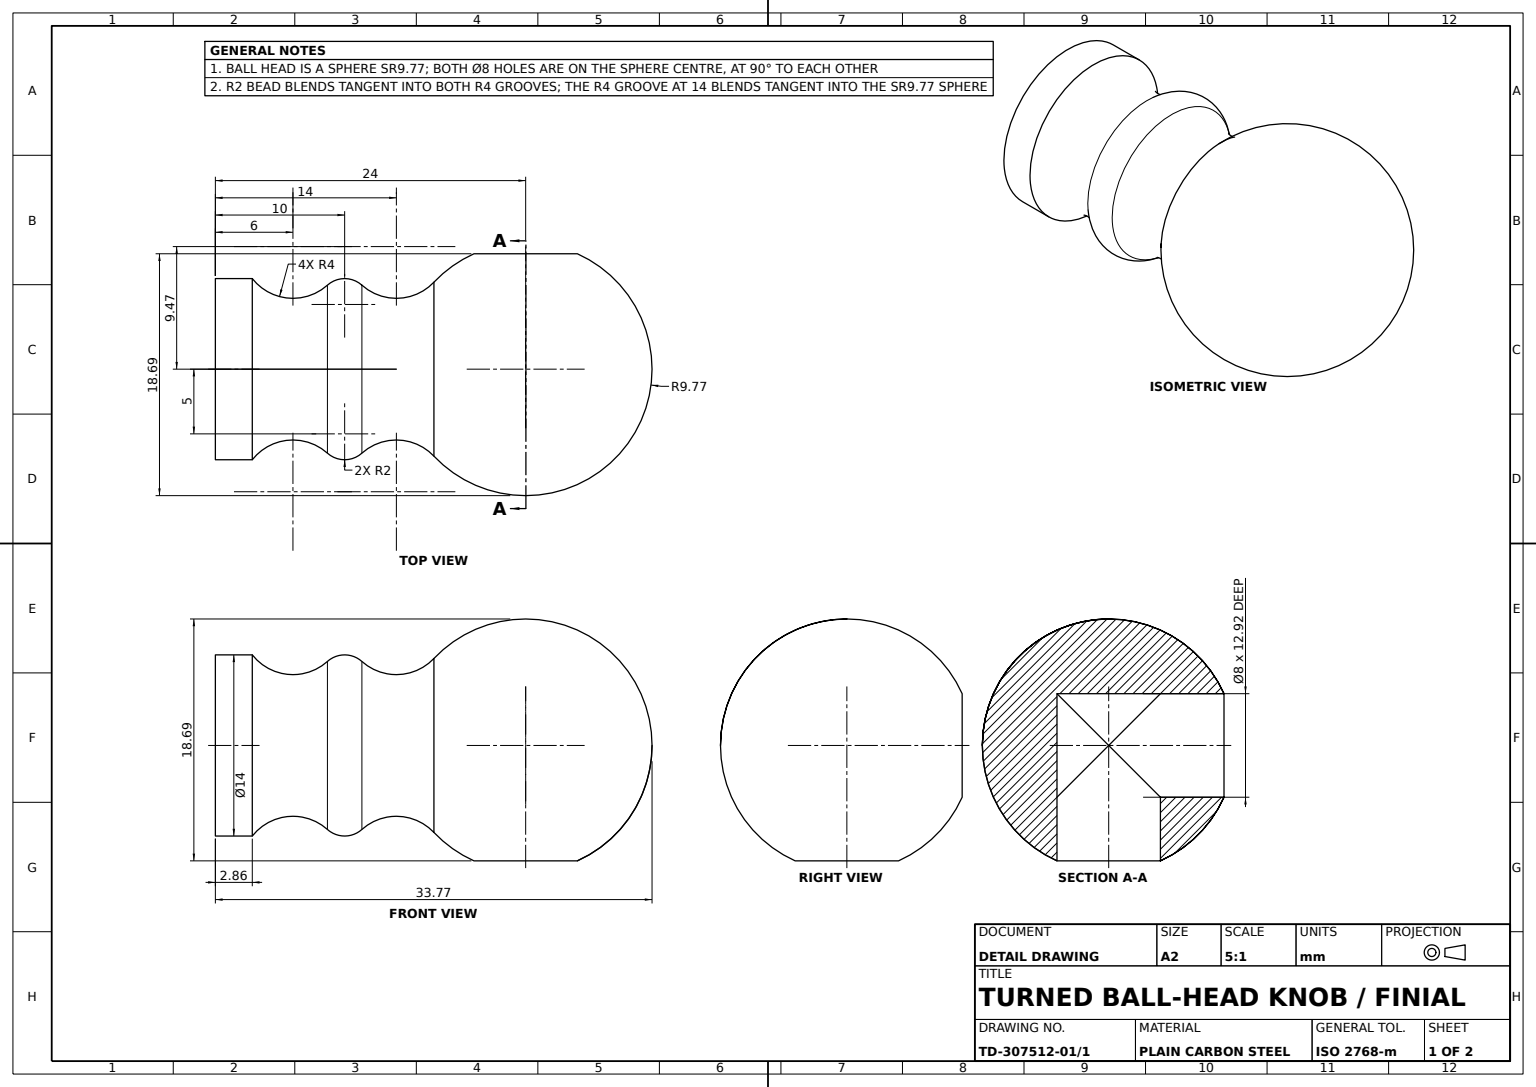
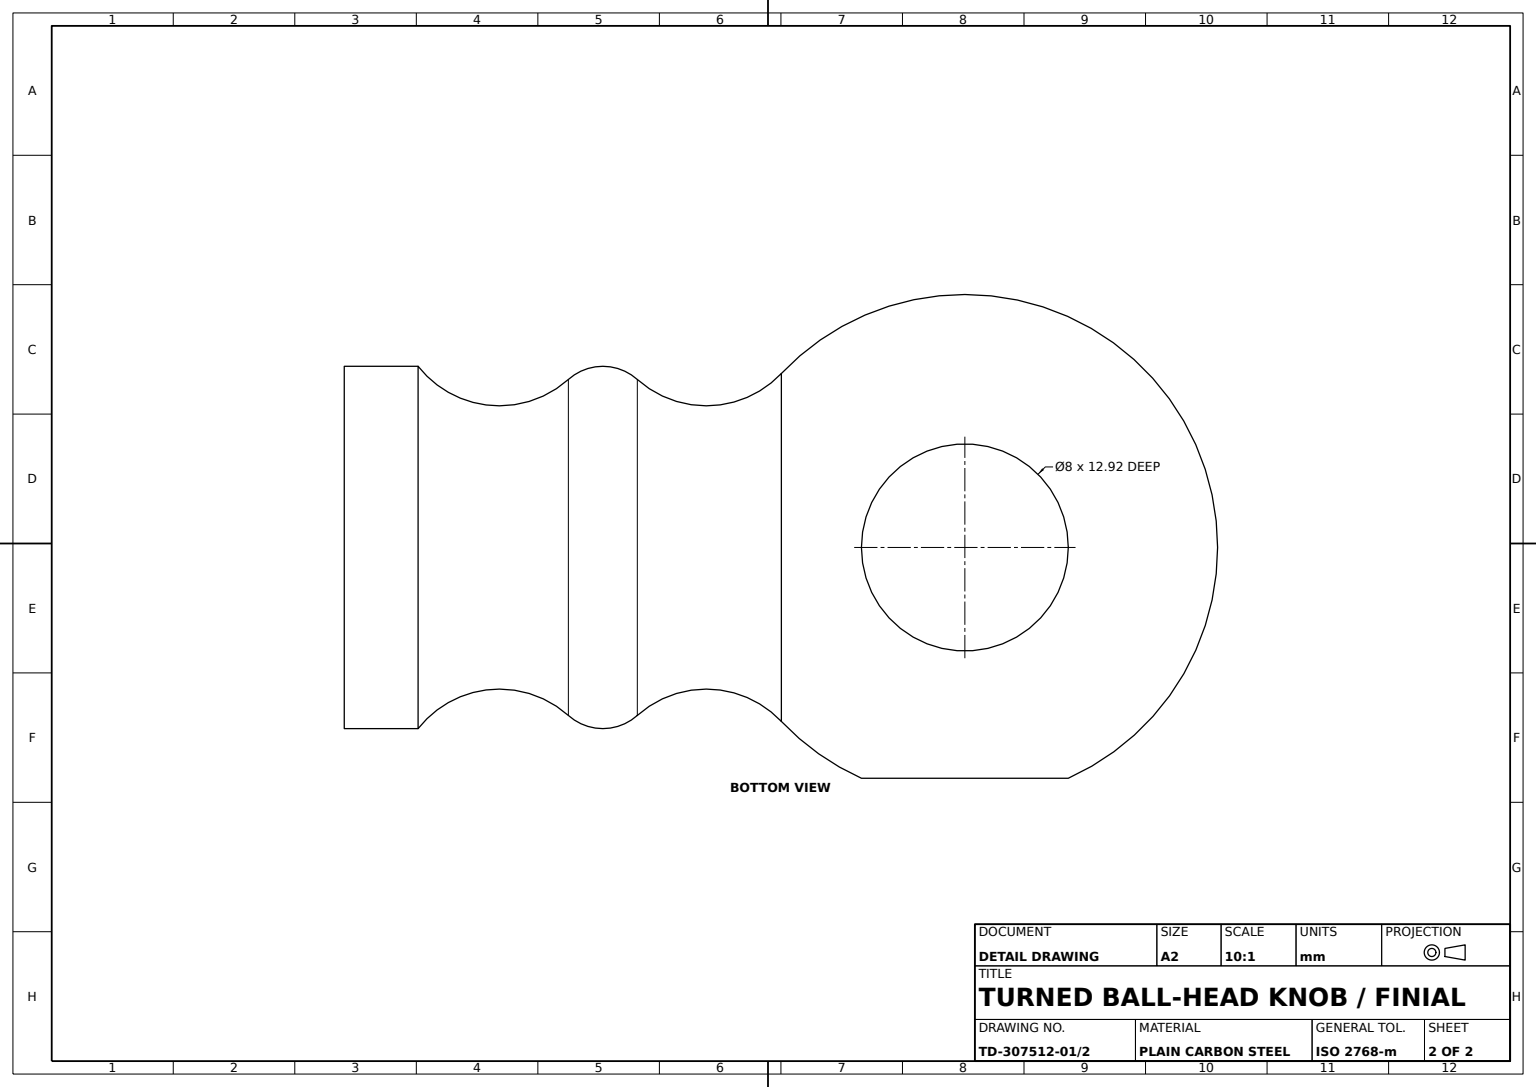
from build123d import *

# Parameters (mm, degrees)
SIDE_CUT_8_DEPTH_4_DEPTH             = 4
SIDE_CUT_8_DEPTH_4_DEPTH_BACK        = 37.492993619
SIDE_CUT_8_SKETCH_RIGHT_PLANE_R      = 4
CROSS_CUT_8_TWO_DIRECTION_DEPTH      = 4
CROSS_CUT_8_TWO_DIRECTION_DEPTH_BACK = 10
CROSS_CUT_8_SKETCH_TOP_PLANE_R       = 4


with BuildPart() as part:
    # Knob Profile Sketch → Knob Body Revolve (revolve)
    with BuildSketch(Plane(origin=(0, 0, 0), x_dir=(1, 0, 0), z_dir=(0, 1, 0))):
        with BuildLine():
            Line((0, 0), (0, 33.773937692))
            ThreePointArc((0, 33.773937692), (9.079795586, 27.617619401), (6.721394325, 16.904035207))
            ThreePointArc((6.721394325, 16.904035207), (5.475561114, 14.165497859), (6.490711985, 11.333333333))
            ThreePointArc((6.490711985, 11.333333333), (7, 10), (6.490711985, 8.666666667))
            ThreePointArc((6.490711985, 8.666666667), (5.487408857, 5.650786662), (7, 2.855394489))
            Line((7, 2.855394489), (7, 0))
            Line((7, 0), (0, 0))
        make_face()
    revolve(axis=Axis((0, 0, 0), (0, 0, -1)))

    # Side Cut _8 Sketch _Right Plane → Side Cut _8 Depth 4 (cut, two sides: drawn at the far end of the back side and taken through both)
    with BuildSketch(Plane(origin=(0, 0, 0), x_dir=(0, 0, -1), z_dir=(1, 0, 0)).offset(-SIDE_CUT_8_DEPTH_4_DEPTH_BACK)):
        with Locations((24, 0)):
            Circle(SIDE_CUT_8_SKETCH_RIGHT_PLANE_R)
    extrude(amount=SIDE_CUT_8_DEPTH_4_DEPTH + SIDE_CUT_8_DEPTH_4_DEPTH_BACK, mode=Mode.SUBTRACT)

    # Cross Cut _8 Sketch _Top Plane → Cross Cut _8 Two-Direction (cut, two sides: drawn at the far end of the back side and taken through both)
    with BuildSketch(Plane(origin=(0, 0, 0), x_dir=(1, 0, 0), z_dir=(0, 1, 0)).offset(-CROSS_CUT_8_TWO_DIRECTION_DEPTH_BACK)):
        with Locations(Location((0, 24, 0), (0, 0, 270))):
            Circle(CROSS_CUT_8_SKETCH_TOP_PLANE_R)
    extrude(amount=CROSS_CUT_8_TWO_DIRECTION_DEPTH + CROSS_CUT_8_TWO_DIRECTION_DEPTH_BACK, mode=Mode.SUBTRACT)


solid = part.part
